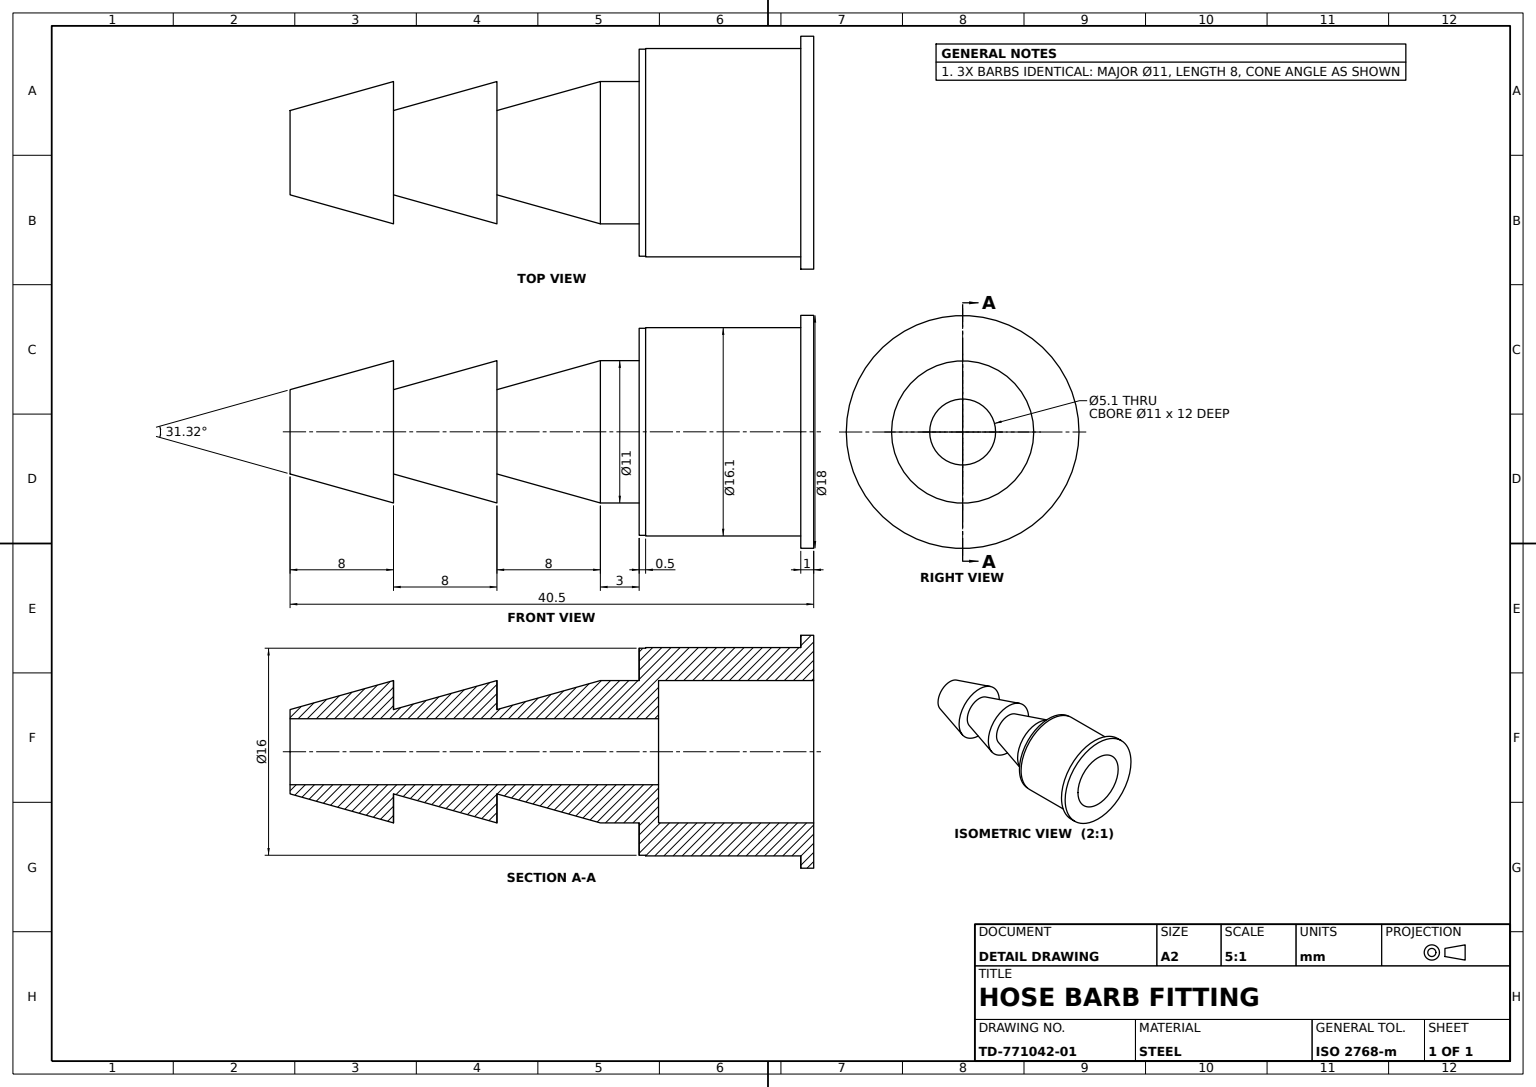
SolidWorks part; units mm, degrees
material "Plain Carbon Steel"
ref_plane "Front Plane" through (0, 0, 0) normal (0, 0, 1) x (1, 0, 0)
ref_plane "Top Plane" through (0, 0, 0) normal (0, 1, 0) x (1, 0, 0)
ref_plane "Right Plane" through (0, 0, 0) normal (1, 0, 0) x (0, 0, -1)
sketch "Flange Sketch" plane through (0, 0, 0) normal (0, 0, 1) x (1, 0, 0)
  circle A0 centre (0, 0) radius 9
  dimension "D1" = 18
extrude "Flange" add sketch "Flange Sketch" along normal blind 1
sketch "Body Sketch" plane through (0, 0, 1) normal (0, 0, 1) x (1, 0, 0)
  circle A0 centre (0, 0) radius 8.05
  dimension "D1" = 16.1
extrude "Body" add sketch "Body Sketch" along normal blind 12
sketch "Shoulder Step Sketch" plane through (0, 0, 13) normal (0, 0, 1) x (1, 0, 0)
  circle A1 centre (0, 0) radius 8
  dimension "D1" = 16
extrude "Shoulder Step" add sketch "Shoulder Step Sketch" along normal blind 0.5
sketch "Neck Sketch" plane through (0, 0, 13.5) normal (0, 0, 1) x (1, 0, 0)
  circle A0 centre (0, 0) radius 5.5
  dimension "D1" = 11
extrude "Neck" add sketch "Neck Sketch" along normal blind 3
sketch "Barb 1 Sketch" plane through (0, 0, 16.5) normal (0, 0, 1) x (1, 0, 0)
  circle A0 centre (0, 0) radius 5.5
  dimension "D1" = 11
extrude "Barb 1" add sketch "Barb 1 Sketch" along normal blind 8 draft 15.66
sketch "Barb 2 Sketch" plane through (0, 0, 24.5) normal (0, 0, 1) x (1, 0, 0)
  circle A0 centre (0, 0) radius 5.5
  dimension "D1" = 11
extrude "Barb 2" add sketch "Barb 2 Sketch" along normal blind 8 draft 15.66
sketch "Barb 3 Sketch" plane through (0, 0, 32.5) normal (0, 0, 1) x (1, 0, 0)
  circle A0 centre (0, 0) radius 5.5
  dimension "D1" = 11
extrude "Barb 3 Tip" add sketch "Barb 3 Sketch" along normal blind 8 draft 15.66
sketch "Inlet Bore Sketch" plane through (0, 0, 0) normal (0, 0, -1) x (-1, 0, 0)
  circle A0 centre (0, 0) radius 5.5
  dimension "D1" = 11
extrude "Inlet Bore" cut sketch "Inlet Bore Sketch" against normal blind 12
sketch "Through Bore Sketch" plane through (0, 0, 12) normal (0, 0, -1) x (-1, 0, 0)
  circle A0 centre (0, 0) radius 2.55
  dimension "D1" = 5.1
extrude "Through Bore" cut sketch "Through Bore Sketch" against normal blind 38
